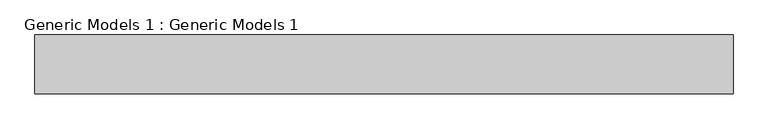
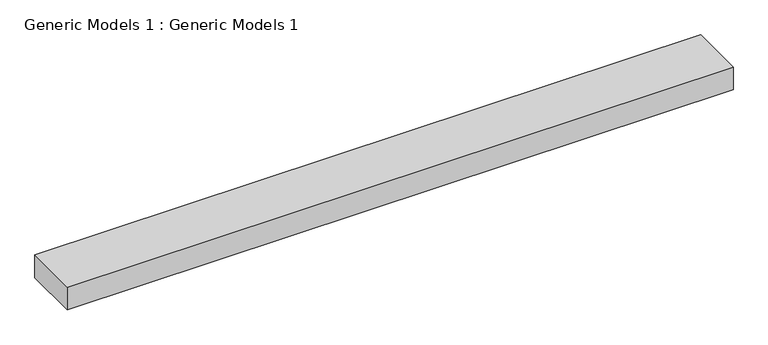
"""IFC4 building model written with IfcOpenShell, lengths in millimetres: proxy geometry, Generic Models 1 : Generic Models 1."""

from ifc_helpers import new_model, si_unit, frame, origin, place, context, project, spatial, polyline, outline, extrude, source, transform, mapped, element, save


def generic_models_1_generic_models_1_44a9a556(model_context):
    return source(origin(), model_context, "Body", "SweptSolid", [
        extrude(outline(polyline([(-4797.9586008, -8059.5844117), (-12049.6586008, -8059.5844117), (-12049.6586008, -7449.9844117), (-4797.9586008, -7449.9844117), (-4797.9586008, -8059.5844117)])), frame((0.0, 0.0, 6137.7541096), z_axis=(0.0, 0.0, 1.0), x_axis=(1.0, 0.0, 0.0)), (0.0, 0.0, 1.0), 263.0458904),
    ])


if __name__ == "__main__":
    model = new_model("IFC4")
    model_context = context("Model", 3, world=origin())
    ifc_project = project(units=[si_unit("LENGTHUNIT", "METRE", prefix="MILLI")], contexts=[model_context])
    site = spatial("IfcSite", under=ifc_project)
    building = spatial("IfcBuilding", under=site)
    placement = place(None, origin())
    generic_models_1_generic_models_1_shape = generic_models_1_generic_models_1_44a9a556(model_context)
    element("IfcBuildingElementProxy", 1, Name="Generic Models 1 : Generic Models 1", ObjectType="Generic Models 1 : Generic Models 1", at=placement, inside=building, context=model_context, shape_type="MappedRepresentation", body=[
        mapped(generic_models_1_generic_models_1_shape, transform((0.0, 0.0, 0.0), x_axis=(1.0, 0.0, 0.0), y_axis=(0.0, 1.0, 0.0), z_axis=(0.0, 0.0, 1.0))),
    ])
    save(model, "model.ifc")

# Revit data of these elements
# Element 1 (IfcBuildingElementProxy, "Generic Models 1 : Generic Models 1")
#   Materials on its faces: "Clad - White"
# Materials
#   "Clad - White": class "Wood", colour RGB 242 242 238, transparency 0, Cost = 0
